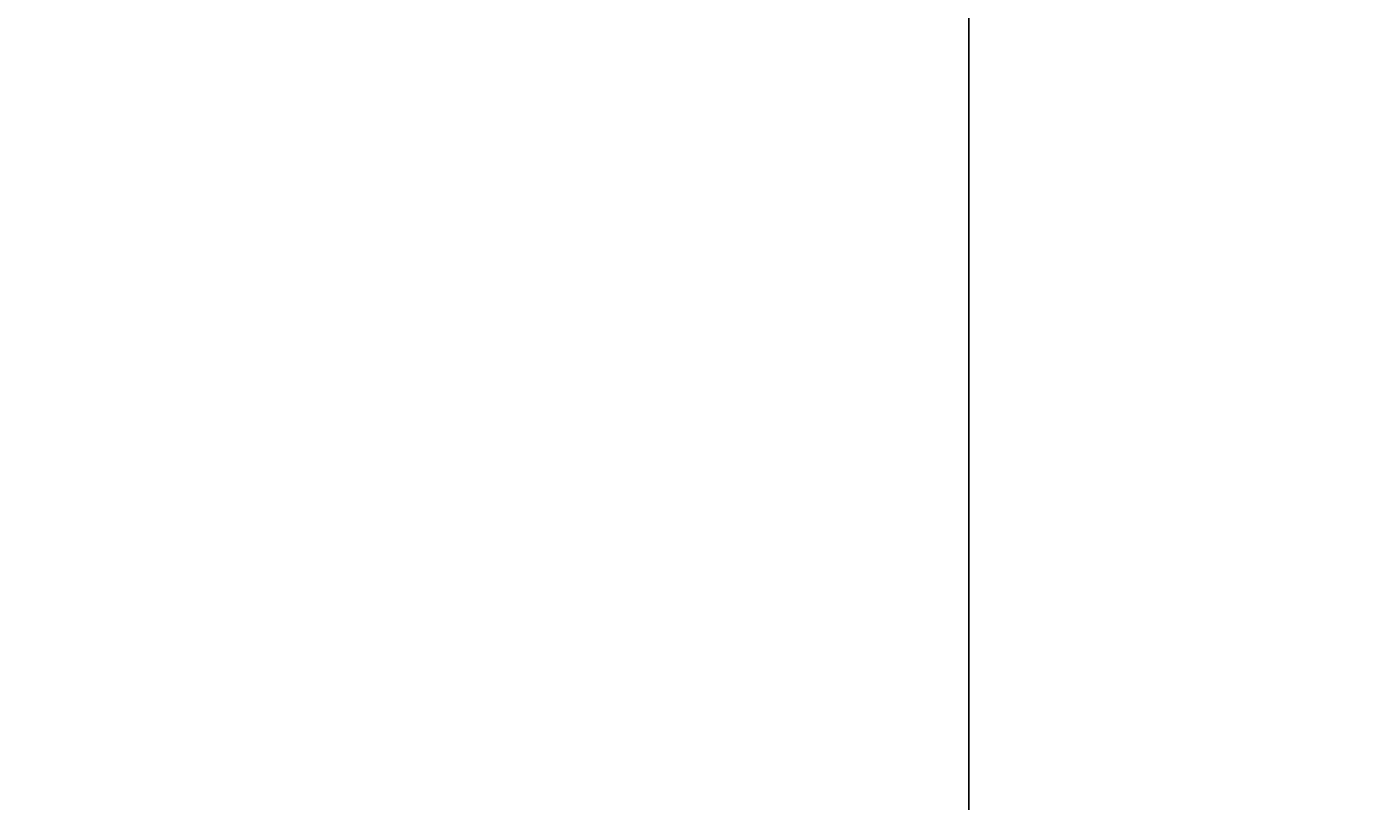
# Model space of a CAD drawing. Units: inches. Extents: x 35362 to 73946, y 43607 to 67532.
# Tile 133 of 134: x 66704 to 67594, y 44948 to 45460. Entities that reach past the tile are written whole.
import ezdxf

# ---------------------------------------------------------------- set-up
doc = ezdxf.new("R2010")
doc.units = ezdxf.units.IN
doc.header["$MEASUREMENT"] = 0
doc.layers.add('A-ANNO-DIMS', color=2, linetype='Continuous', lineweight=18)
doc.styles.get("Standard").update_dxf_attribs({"font": 'arial.ttf'})
doc.dimstyles.get("Standard").update_dxf_attribs({"dimtxt": 0.18, "dimasz": 0.18, "dimexe": 0.18, "dimexo": 0.0625, "dimgap": 0.09, "dimtad": 0, "dimtih": 1, "dimtoh": 1, "dimdec": 4, "dimzin": 0, "dimdsep": 46, "dimtxsty": 'Standard', "dimcen": 0.09, "dimadec": 0, "dimazin": 0, "dimtfac": 1, "dimtdec": 4, "dimtofl": 0, "dimtmove": 0, "dimatfit": 3, "dimfxl": 1, "dimtolj": 1, "dimtzin": 0, "dimarcsym": 0})

# ---------------------------------------------------------------- blocks, each defined once
blk = doc.blocks.new('*D5')
at = {"layer": 'A-ANNO-DIMS', "color": 0, "lineweight": -2, "transparency": 16777216}
for p, q in [((37121.949085, 46919.318283), (37121.949085, 43606.678996)), ((69871.496302, 45449.831951), (69871.496302, 43606.678996)), ((37122.129085, 43606.858996), (53496.2943647142, 43606.858996)), ((69871.316302, 43606.858996), (53497.15102228581, 43606.858996))]:
    blk.add_line(p, q, dxfattribs=at)
at = {"layer": 'A-ANNO-DIMS', "color": 0, "transparency": 16777216}
for points in [[(37122.129085, 43606.888996), (37122.129085, 43606.828996), (37121.949085, 43606.858996)], [(69871.316302, 43606.888996), (69871.316302, 43606.828996), (69871.496302, 43606.858996)]]:
    blk.add_solid(points, dxfattribs=at)
at = {"layer": 'Defpoints', "color": 0, "transparency": 16777216}
for p in [(37121.949085, 46919.380783), (69871.496302, 45449.894451), (69871.496302, 43606.858996)]:
    blk.add_point(p, dxfattribs=at)
at = {"layer": 'A-ANNO-DIMS', "color": 0, "transparency": 16777216, "insert": (53496.7226935, 43606.858996), "char_height": 0.18, "attachment_point": 5}
blk.add_mtext('\\A1;32750', dxfattribs=at)
blk = doc.blocks.new('*D38')
at = {"layer": 'A-ANNO-DIMS', "color": 0, "lineweight": -2, "transparency": 16777216}
for p, q in [((68483.500128, 45449.831951), (68483.500128, 43606.678996)), ((62090.58505699999, 45366.796496), (62090.58505699999, 43606.678996)), ((62090.76505699999, 43606.858996), (65286.57828827081, 43606.858996)), ((68483.320128, 43606.858996), (65287.5068967292, 43606.858996))]:
    blk.add_line(p, q, dxfattribs=at)
at = {"layer": 'A-ANNO-DIMS', "color": 0, "transparency": 16777216}
for points in [[(62090.76505699999, 43606.888996), (62090.76505699999, 43606.828996), (62090.58505699999, 43606.858996)], [(68483.320128, 43606.888996), (68483.320128, 43606.828996), (68483.500128, 43606.858996)]]:
    blk.add_solid(points, dxfattribs=at)
at = {"layer": 'Defpoints', "color": 0, "transparency": 16777216}
for p in [(68483.500128, 45449.894451), (62090.58505699999, 45366.858996), (68483.500128, 43606.858996)]:
    blk.add_point(p, dxfattribs=at)
at = {"layer": 'A-ANNO-DIMS', "color": 0, "transparency": 16777216, "insert": (65287.0425925, 43606.858996), "char_height": 0.18, "attachment_point": 5}
blk.add_mtext('\\A1;6392.9', dxfattribs=at)
blk = doc.blocks.new('*D65')
at = {"layer": 'A-ANNO-DIMS', "color": 0, "lineweight": -2, "transparency": 16777216}
for p, q in [((65336.01600799999, 61293.223552), (65336.01600799999, 43606.678996)), ((67326.639741, 61293.223552), (67326.639741, 43606.678996)), ((65336.19600799999, 43606.858996), (66330.87277900206, 43606.858996)), ((67326.45974100001, 43606.858996), (66331.78296999796, 43606.858996))]:
    blk.add_line(p, q, dxfattribs=at)
at = {"layer": 'A-ANNO-DIMS', "color": 0, "transparency": 16777216}
for points in [[(65336.19600799999, 43606.888996), (65336.19600799999, 43606.828996), (65336.01600799999, 43606.858996)], [(67326.45974100001, 43606.888996), (67326.45974100001, 43606.828996), (67326.639741, 43606.858996)]]:
    blk.add_solid(points, dxfattribs=at)
at = {"layer": 'Defpoints', "color": 0, "transparency": 16777216}
for p in [(65336.01600799999, 61293.286052), (67326.639741, 61293.286052), (67326.639741, 43606.858996)]:
    blk.add_point(p, dxfattribs=at)
at = {"layer": 'A-ANNO-DIMS', "color": 0, "transparency": 16777216, "insert": (66331.32787450001, 43606.858996), "char_height": 0.18, "attachment_point": 5}
blk.add_mtext('\\A1;1990.6', dxfattribs=at)
blk = doc.blocks.new('*D68')
at = {"layer": 'A-ANNO-DIMS', "color": 0, "lineweight": -2, "transparency": 16777216}
for p, q in [((68320.870762, 54372.885224), (68320.870762, 43606.678996)), ((61240.907336, 53351.466162), (61240.907336, 43606.678996)), ((61241.08733599999, 43606.858996), (64780.42646373397, 43606.858996)), ((68320.69076200001, 43606.858996), (64781.35163426603, 43606.858996))]:
    blk.add_line(p, q, dxfattribs=at)
at = {"layer": 'A-ANNO-DIMS', "color": 0, "transparency": 16777216}
for points in [[(61241.08733599999, 43606.888996), (61241.08733599999, 43606.828996), (61240.907336, 43606.858996)], [(68320.69076200001, 43606.888996), (68320.69076200001, 43606.828996), (68320.870762, 43606.858996)]]:
    blk.add_solid(points, dxfattribs=at)
at = {"layer": 'Defpoints', "color": 0, "transparency": 16777216}
for p in [(68320.870762, 54372.947724), (61240.907336, 53351.52866199999), (68320.870762, 43606.858996)]:
    blk.add_point(p, dxfattribs=at)
at = {"layer": 'A-ANNO-DIMS', "color": 0, "transparency": 16777216, "insert": (64780.889049, 43606.858996), "char_height": 0.18, "attachment_point": 5}
blk.add_mtext('\\A1;7080.0', dxfattribs=at)

msp = doc.modelspace()

# ---------------------------------------------------------------- dimensions: what is measured, and where the dimension line sits
at = {"layer": 'A-ANNO-DIMS'}
for base, p1, p2, override, picture, middle in [((67326.639741, 43606.858996), (65336.01600799999, 61293.286052), (67326.639741, 61293.286052), {"dimdec": 1, "dimlfac": 1, "dimrnd": 0, "dimzin": 0, "dimdsep": 46, "dimlunit": 2}, '*D65', (66331.32787450001, 43606.858996)), ((68320.870762, 43606.858996), (61240.907336, 53351.52866199999), (68320.870762, 54372.947724), {"dimdec": 1, "dimlfac": 1, "dimrnd": 0, "dimzin": 0, "dimdsep": 46, "dimlunit": 2}, '*D68', (64780.889049, 43606.858996)), ((69871.496302, 43606.858996), (37121.949085, 46919.380783), (69871.496302, 45449.894451), {"dimdec": 0, "dimlfac": 1, "dimrnd": 0, "dimzin": 0, "dimdsep": 46, "dimlunit": 2}, '*D5', (53496.7226935, 43606.858996)), ((68483.500128, 43606.858996), (62090.58505699999, 45366.858996), (68483.500128, 45449.894451), {"dimdec": 1, "dimlfac": 1, "dimrnd": 0, "dimzin": 0, "dimdsep": 46, "dimlunit": 2}, '*D38', (65287.0425925, 43606.858996))]:
    dim = msp.add_linear_dim(base=base, p1=p1, p2=p2, dimstyle='Standard', override=override, dxfattribs=at)
    dim.commit()
    dim.dimension.update_dxf_attribs({"geometry": picture, "text_midpoint": middle})

doc.saveas('drawing.dxf')
